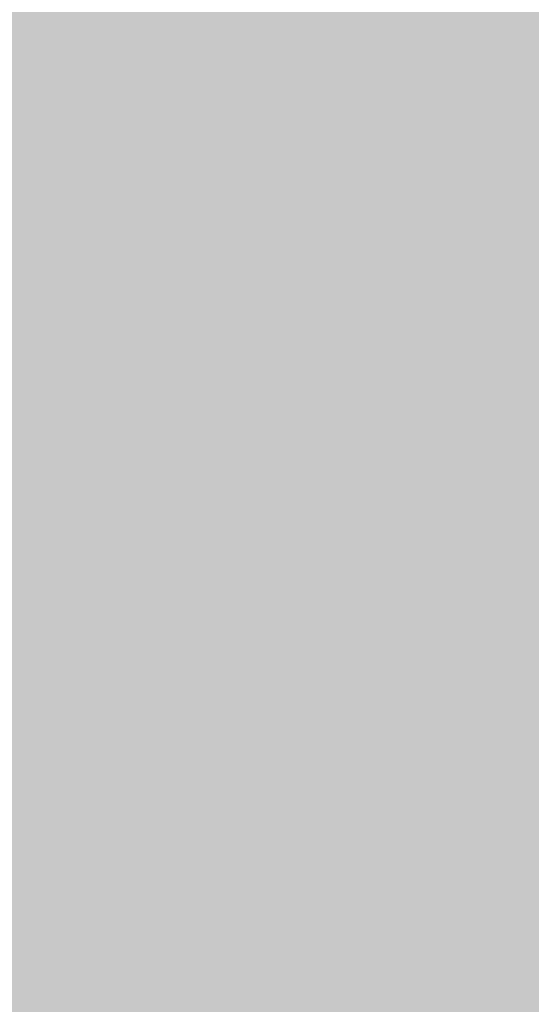
# Model space of a CAD drawing. Units: inches. Extents: x 2083 to 3317, y 1141 to 2115.
# Tile 198 of 256: x 3126.6699 to 3126.939, y 1263.6134 to 1264.1307. Entities that reach past the tile are written whole.
import ezdxf

# ---------------------------------------------------------------- set-up
doc = ezdxf.new("R2010")
doc.units = ezdxf.units.IN
doc.layers.add('A-ANNO-DIMS', color=2, linetype='Continuous', lineweight=18)
doc.layers.add('A-WALL-PATT', color=251, linetype='Continuous', lineweight=13, true_color=0x636466)
doc.styles.get("Standard").update_dxf_attribs({"font": 'arial.ttf'})
doc.dimstyles.new('ISO-25', dxfattribs={"dimtxt": 12, "dimasz": 12, "dimexe": 1.25, "dimexo": 0.625, "dimtad": 1, "dimlunit": 3, "dimtxsty": 'Standard', "dimcen": 2.5, "dimadec": 0, "dimazin": 0, "dimtfac": 1, "dimtmove": 0, "dimatfit": 3, "dimfxl": 1, "dimarcsym": 0})

# ---------------------------------------------------------------- blocks, each defined once
blk = doc.blocks.new('*D26')
at = {"layer": 'A-ANNO-DIMS', "color": 0, "lineweight": -2, "transparency": 16777216}
for p, q in [((3088.98584, 1274.91509), (3088.98584, 1270.95196)), ((3111.24004, 1274.91509), (3111.24004, 1270.95196)), ((3076.98584, 1272.20196), (2840.26245, 1272.20196)), ((3111.24004, 1272.20196), (3088.98584, 1272.20196)), ((3123.24004, 1272.20196), (3135.24004, 1272.20196))]:
    blk.add_line(p, q, dxfattribs=at)
at = {"layer": 'A-ANNO-DIMS', "color": 0, "transparency": 16777216}
for points in [[(3076.98584, 1274.20196), (3076.98584, 1270.20196), (3088.98584, 1272.20196)], [(3123.24004, 1274.20196), (3123.24004, 1270.20196), (3111.24004, 1272.20196)]]:
    blk.add_solid(points, dxfattribs=at)
at = {"layer": 'Defpoints', "color": 0, "transparency": 16777216}
for p in [(3088.98584, 1275.54009), (3111.24004, 1275.54009), (3088.98584, 1272.20196)]:
    blk.add_point(p, dxfattribs=at)
at = {"layer": 'A-ANNO-DIMS', "color": 0, "transparency": 16777216, "insert": (2952.62415, 1279.0316), "char_height": 12, "attachment_point": 5}
blk.add_mtext('NIGHTSTAND 1\'-10 1/2" TYP.', dxfattribs=at)
blk = doc.blocks.new('*D27')
at = {"layer": 'A-ANNO-DIMS', "color": 0, "lineweight": -2, "transparency": 16777216}
for p, q in [((3114.57817, 1309.79428), (3114.57817, 1321.79428)), ((3111.86504, 1297.79428), (3115.82817, 1297.79428)), ((3114.57817, 1297.79428), (3114.57817, 1275.54009)), ((3111.86504, 1275.54009), (3115.82817, 1275.54009)), ((3114.57817, 1263.54009), (3114.57817, 1140.98859))]:
    blk.add_line(p, q, dxfattribs=at)
at = {"layer": 'A-ANNO-DIMS', "color": 0, "transparency": 16777216}
for points in [[(3112.57817, 1309.79428), (3116.57817, 1309.79428), (3114.57817, 1297.79428)], [(3112.57817, 1263.54009), (3116.57817, 1263.54009), (3114.57817, 1275.54009)]]:
    blk.add_solid(points, dxfattribs=at)
at = {"layer": 'Defpoints', "color": 0, "transparency": 16777216}
for p in [(3111.24004, 1297.79428), (3111.24004, 1275.54009), (3114.57817, 1275.54009)]:
    blk.add_point(p, dxfattribs=at)
at = {"layer": 'A-ANNO-DIMS', "color": 0, "transparency": 16777216, "insert": (3107.74853, 1196.26434), "char_height": 12, "attachment_point": 5, "rotation": 90}
blk.add_mtext('1\'-10 1/2" TYP.', dxfattribs=at)

msp = doc.modelspace()

# ---------------------------------------------------------------- hatches: boundary and pattern name
at = {"layer": 'A-WALL-PATT'}
h = msp.add_hatch(color=256, dxfattribs=at)
h.dxf.hatch_style = 1
h.paths.add_polyline_path([(3126.95978, 2020.76136), (2748.95978, 2020.76136), (2604.95978, 2020.76136), (2226.95978, 2020.76136), (2226.95978, 1702.76136), (2466.95978, 1702.76136), (2466.95978, 1582.76136), (2418.95978, 1582.76136), (2418.95978, 1477.76136), (2226.95978, 1477.76136), (2226.95978, 1263.26136), (2544.95978, 1263.26136), (2544.95978, 1411.76136), (2604.95978, 1411.76136), (2685.95978, 1411.76136), (2685.95978, 1420.76136), (2604.95978, 1420.76136), (2604.95978, 1573.76136), (2604.95978, 1702.76136), (2604.95978, 2011.76136), (2748.95978, 2011.76136), (2748.95978, 1702.76136), (2862.95978, 1702.76136), (2862.95978, 1621.76136), (2871.95978, 1621.76136), (2871.95978, 1702.76136), (2883.95978, 1702.76136), (2883.95978, 1706.93946, -0.026459), (2883.95978, 1711.76136), (2757.95978, 1711.76136), (2757.95978, 1807.76136), (2787.95978, 1807.76136), (2787.95978, 1812.26136), (2757.95978, 1812.26136), (2757.95978, 2011.76136), (2877.95978, 2011.76136), (2877.95978, 1812.26136), (2847.95978, 1812.26136), (2847.95978, 1807.76136), (2889.83574, 1807.76136), (2889.83574, 1812.26136), (2882.45978, 1812.26136), (2882.45978, 2011.76136), (3117.95978, 2011.76136), (3117.95978, 1812.26136), (2937.83574, 1812.26136), (2937.83574, 1807.76136), (2995.70978, 1807.76136), (2995.70978, 1796.11767), (3000.20978, 1796.11767), (3000.20978, 1807.76136), (3117.95978, 1807.76136), (3117.95978, 1711.76136), (3000.20978, 1711.76136), (3000.20978, 1760.11767), (2998.5727, 1760.11767, -0.020711), (2995.70978, 1760.11767), (2995.70978, 1711.76136), (2931.95978, 1711.76136), (2931.95978, 1702.76136), (3126.95978, 1702.76136)])
h.paths.add_polyline_path([(2471.45978, 2011.76136), (2471.45978, 1810.01136), (2462.71694, 1810.01136), (2462.71694, 1805.51136), (2505.95978, 1805.51136), (2505.95978, 1810.01136), (2475.95978, 1810.01136), (2475.95978, 2011.76136), (2595.95978, 2011.76136), (2595.95978, 1810.01136), (2565.95978, 1810.01136), (2565.95978, 1805.51136), (2595.95978, 1805.51136), (2595.95978, 1711.76136), (2235.95978, 1711.76136), (2235.95978, 1805.51136), (2353.70978, 1805.51136), (2353.70978, 1796.05416), (2358.20978, 1796.05416), (2358.20978, 1805.51136), (2414.71694, 1805.51136), (2414.71694, 1810.01136), (2235.95978, 1810.01136), (2235.95978, 2011.76136)], flags=16)
h.paths.add_polyline_path([(2270.20473, 1994.61001), (2270.20473, 1970.61001), (2246.20473, 1970.61001), (2246.20473, 1994.61001)], flags=0)
edge = h.paths.add_edge_path(flags=0)
edge.add_ellipse((2332.02739, 1899.79818), major_axis=(-3.04299, 3.04299), ratio=0.1682525, start_angle=-161.33217, end_angle=-156.30711, ccw=False)
edge.add_ellipse((2333.08204, 1898.74353), major_axis=(-1.05465, 1.05465), ratio=0.4535321, start_angle=-123.37102, end_angle=-94.15911)
edge = h.paths.add_edge_path(flags=0)
edge.add_ellipse((2332.02739, 1968.87629), major_axis=(3.04299, 3.04299), ratio=0.1682525, start_angle=18.66783, end_angle=23.69289)
edge.add_spline(control_points=[(2332.9256, 1970.6911), (2332.22677, 1970.3361), (2330.89371, 1969.65891), (2328.41308, 1970.93214), (2327.20393, 1967.74871), (2324.7096, 1969.95559), (2322.53282, 1967.01235), (2320.01285, 1971.29581), (2317.68031, 1968.15784), (2316.04053, 1967.10205), (2315.4269, 1966.8096)], knot_values=[0, 0, 0, 0, 2.267059, 4.324559, 6.685584, 8.878641, 11.121502, 14.300359, 17.755284, 19.732645, 19.732645, 19.732645, 19.732645], degree=3, periodic=0)
edge.add_ellipse((2332.02739, 1968.87629), major_axis=(3.04299, 3.04299), ratio=0.1682525, start_angle=18.66783, end_angle=23.69289, ccw=False)
edge.add_ellipse((2333.08204, 1969.93094), major_axis=(1.05465, 1.05465), ratio=0.4535321, start_angle=56.62898, end_angle=85.84089, ccw=False)
edge = h.paths.add_edge_path(flags=0)
edge.add_spline(control_points=[(2296.42829, 1967.98791), (2293.6278, 1965.33631), (2287.70362, 1959.72709), (2299.74386, 1949.9957), (2294.53259, 1935.66853), (2290.57323, 1920.60351), (2293.39412, 1909.97369), (2296.18541, 1904.96654)], knot_values=[0.099185, 0.099185, 0.099185, 0.099185, 0.345301, 0.619822, 0.982653, 1.386093, 1.810555, 1.810555, 1.810555, 1.810555], degree=3, periodic=0)
edge.add_spline(control_points=[(2296.18541, 1904.96654), (2297.38358, 1902.6193), (2298.00097, 1901.94931), (2298.55297, 1901.46815)], knot_values=[0.006246, 0.006246, 0.006246, 0.006246, 0.055476, 0.055476, 0.055476, 0.055476], degree=3, periodic=0)
edge.add_spline(control_points=[(2298.55297, 1901.46815), (2297.25861, 1900.92322), (2295.22529, 1900.23213), (2293.06023, 1900.61421), (2292.10142, 1900.78841), (2292.08958, 1900.79057)], knot_values=[0.312835, 0.312835, 0.312835, 0.312835, 0.40178, 0.474987, 0.475903, 0.475903, 0.475903, 0.475903], degree=3, periodic=0)
edge.add_arc((2292.79365, 1904.66411), 3.93701, 215.4209, 259.69818, ccw=False)
edge.add_spline(control_points=[(2289.58531, 1902.3823), (2289.47665, 1902.53509), (2289.36848, 1902.68804), (2289.26086, 1902.84117)], knot_values=[0.102872, 0.102872, 0.102872, 0.102872, 0.116896, 0.116896, 0.116896, 0.116896], degree=3, periodic=0)
edge.add_spline(control_points=[(2289.26086, 1902.84117), (2288.6866, 1902.55019), (2287.64005, 1902.0199), (2285.88134, 1901.87395), (2283.85297, 1901.50435), (2281.71999, 1899.71054), (2278.46699, 1899.49294), (2276.15714, 1901.8832), (2272.25895, 1899.80407), (2267.77761, 1901.84318), (2262.24388, 1900.18403), (2257.41493, 1901.78206), (2254.31837, 1900.72612), (2253.17828, 1900.33734)], knot_values=[0, 0, 0, 0, 1.907977, 3.477176, 5.261074, 7.972851, 11.680248, 13.717921, 16.939592, 22.789562, 27.502503, 33.595215, 37.145618, 37.145618, 37.145618, 37.145618], degree=3, periodic=0)
edge.add_line((2253.17828, 1900.33734), (2250.24424, 1902.84117))
edge.add_line((2250.24424, 1902.84117), (2250.24424, 1965.8333))
edge.add_line((2250.24424, 1965.8333), (2253.17828, 1968.33712))
edge.add_spline(control_points=[(2253.17828, 1968.33712), (2254.31837, 1967.94835), (2257.41493, 1966.89241), (2262.24388, 1968.49043), (2267.77761, 1966.83128), (2271.52673, 1968.53722), (2273.87591, 1967.82829), (2274.2067, 1967.72764)], knot_values=[0, 0, 0, 0, 0.09018, 0.244935, 0.364644, 0.513233, 0.537855, 0.537855, 0.537855, 0.537855], degree=3, periodic=0)
edge.add_arc((2274.35289, 1963.79335), 3.93701, 72.05113, 92.12795, ccw=False)
edge.add_arc((2281.29693, 1985.23), 18.5963, 252.051134, 288.565722)
edge.add_arc((2292.31672, 1956.02888), 12.64608, 71.026788, 113.778218, ccw=False)
edge = h.paths.add_edge_path(flags=0)
edge.add_spline(control_points=[(2274.89941, 1951.85619), (2275.06616, 1951.61659), (2275.23269, 1951.37659), (2275.39799, 1951.13585)], knot_values=[1.409916, 1.409916, 1.409916, 1.409916, 1.43159, 1.43159, 1.43159, 1.43159], degree=3, periodic=0)
edge.add_spline(control_points=[(2275.39799, 1951.13585), (2275.79211, 1950.56189), (2276.17923, 1949.98377), (2276.54555, 1949.3971)], knot_values=[1.358238, 1.358238, 1.358238, 1.358238, 1.409916, 1.409916, 1.409916, 1.409916], degree=3, periodic=0)
edge.add_line((2276.54555, 1949.3971), (2277.43729, 1947.86218))
edge.add_spline(control_points=[(2277.43729, 1947.86218), (2276.30383, 1945.67311), (2274.6397, 1942.42688), (2274.63161, 1938.0939), (2272.79912, 1930.85155), (2274.35643, 1943.89705), (2275.94768, 1947.92336), (2276.54555, 1949.3971)], knot_values=[0.005632, 0.005632, 0.005632, 0.005632, 0.186014, 0.266002, 0.357087, 0.59639, 0.739732, 0.739732, 0.739732, 0.739732], degree=3, periodic=0)
edge.add_spline(control_points=[(2276.54555, 1949.3971), (2276.17923, 1949.98377), (2275.79211, 1950.56189), (2275.39799, 1951.13585)], knot_values=[1.358238, 1.358238, 1.358238, 1.358238, 1.409916, 1.409916, 1.409916, 1.409916], degree=3, periodic=0)
edge.add_spline(control_points=[(2275.39799, 1951.13585), (2274.9425, 1950.08045), (2274.20776, 1948.02527), (2273.9346, 1944.85148), (2272.46853, 1937.62749), (2273.46622, 1945.69647), (2274.70062, 1951.05947), (2274.89941, 1951.85619)], knot_values=[0.104364, 0.104364, 0.104364, 0.104364, 0.189636, 0.269624, 0.36071, 0.600013, 0.644622, 0.644622, 0.644622, 0.644622], degree=3, periodic=0)
h.paths.add_polyline_path([(2269.16751, 1963.12757, -0.357527), (2268.17063, 1960.97637, -0.092561), (2268.17063, 1939.43632, -0.357527), (2269.16751, 1937.28512, -0.357527), (2267.01631, 1938.282, -0.164785), (2254.68558, 1938.282, -0.357527), (2252.53438, 1937.28512, -0.357527), (2253.53126, 1939.43632, -0.092561), (2253.53126, 1960.97637, -0.357527), (2252.53438, 1963.12757, -0.357527), (2254.68558, 1962.13069, -0.164785), (2267.01631, 1962.13069, -0.357527)], flags=0)
h.paths.add_polyline_path([(2248.87407, 1967.8018), (2248.87407, 1957.02771), (2249.45778, 1957.02771), (2249.45778, 1911.64676), (2248.87407, 1911.64676), (2248.87407, 1900.87267), (2246.51186, 1900.87267, 0.197327), (2244.14966, 1902.45687), (2244.14966, 1966.21759, 0.197327), (2246.51186, 1967.8018)], flags=0)
h.paths.add_polyline_path([(2269.16751, 1931.38934, -0.357527), (2268.17063, 1929.23814, -0.092561), (2268.17063, 1907.6981, -0.357527), (2269.16751, 1905.54689, -0.357527), (2267.01631, 1906.54377, -0.164785), (2254.68558, 1906.54377, -0.357527), (2252.53438, 1905.54689, -0.357527), (2253.53126, 1907.6981, -0.092561), (2253.53126, 1929.23814, -0.357527), (2252.53438, 1931.38934, -0.357527), (2254.68558, 1930.39246, -0.164785), (2267.01631, 1930.39246, -0.357527)], flags=0)
edge = h.paths.add_edge_path(flags=0)
edge.add_spline(control_points=[(2276.19686, 1906.7237), (2276.16814, 1909.02893), (2276.11405, 1913.37185), (2270.59842, 1924.92498), (2273.90517, 1919.01278), (2275.92171, 1916.26206), (2275.47457, 1912.40215), (2277.25787, 1910.38062), (2276.69604, 1908.22504), (2276.64622, 1906.81302), (2276.61782, 1906.00841)], knot_values=[0, 0, 0, 0, 8.61026, 16.221274, 18.843057, 23.804898, 27.440828, 29.356102, 31.203478, 33.650687, 33.650687, 33.650687, 33.650687], degree=3, periodic=0)
edge.add_spline(control_points=[(2276.61782, 1906.00841), (2276.62331, 1905.62414), (2276.49774, 1904.62866), (2275.44178, 1903.85473), (2274.93731, 1903.08045), (2274.85908, 1902.84117)], knot_values=[0.156488, 0.156488, 0.156488, 0.156488, 0.184398, 0.231376, 0.250598, 0.250598, 0.250598, 0.250598], degree=3, periodic=0)
edge.add_line((2274.85908, 1902.84117), (2276.50598, 1902.84117))
edge.add_spline(control_points=[(2276.50598, 1902.84117), (2276.78831, 1903.08494), (2277.66507, 1904.1252), (2278.24954, 1904.34074), (2277.65387, 1908.52739), (2278.15567, 1906.22781), (2278.10046, 1905.28595), (2278.84667, 1904.06901), (2277.85679, 1903.41495), (2277.87419, 1902.99105), (2277.90356, 1902.84117)], knot_values=[0.059574, 0.059574, 0.059574, 0.059574, 0.080753, 0.103741, 0.16972, 0.176036, 0.207137, 0.240474, 0.262341, 0.27366, 0.27366, 0.27366, 0.27366], degree=3, periodic=0)
edge.add_line((2277.90356, 1902.84117), (2280.02983, 1902.84117))
edge.add_spline(control_points=[(2280.02983, 1902.84117), (2279.88822, 1903.0884), (2279.49926, 1903.98155), (2280.15228, 1905.93935), (2278.10362, 1909.65776), (2279.76239, 1907.18529), (2280.3279, 1904.87486), (2280.48511, 1903.48959), (2281.46327, 1903.24943), (2281.75834, 1902.9365), (2281.83404, 1902.84117)], knot_values=[0.013856, 0.013856, 0.013856, 0.013856, 0.034874, 0.088867, 0.107879, 0.126738, 0.158714, 0.193757, 0.217487, 0.226722, 0.226722, 0.226722, 0.226722], degree=3, periodic=0)
edge.add_spline(control_points=[(2281.83404, 1902.84117), (2281.78753, 1902.8267), (2281.64702, 1902.78299), (2281.39553, 1902.85949), (2281.08808, 1902.98524), (2280.72068, 1903.0609), (2280.33345, 1903.02573), (2280.12477, 1902.89888), (2280.02983, 1902.84117)], knot_values=[0, 0, 0, 0, 0.14413, 0.435517, 0.749276, 1.153046, 1.548371, 1.878348, 1.878348, 1.878348, 1.878348], degree=3, periodic=0)
edge.add_line((2280.02983, 1902.84117), (2277.90356, 1902.84117))
edge.add_spline(control_points=[(2277.90356, 1902.84117), (2277.89286, 1902.79586), (2277.8654, 1902.67964), (2277.60748, 1902.68748), (2277.27405, 1902.8007), (2276.83792, 1902.61977), (2276.58381, 1902.78926), (2276.50598, 1902.84117)], knot_values=[0, 0, 0, 0, 0.127189, 0.326199, 0.628009, 1.24357, 1.515331, 1.515331, 1.515331, 1.515331], degree=3, periodic=0)
edge.add_line((2276.50598, 1902.84117), (2274.85908, 1902.84117))
edge.add_spline(control_points=[(2274.85908, 1902.84117), (2274.81444, 1902.89859), (2274.72513, 1903.01345), (2274.49348, 1903.11897), (2274.24429, 1902.96054), (2273.93712, 1903.18494), (2273.61404, 1902.98314), (2273.40832, 1902.88304), (2273.32225, 1902.84117)], knot_values=[0, 0, 0, 0, 0.21843, 0.436957, 0.687977, 0.990379, 1.398396, 1.69185, 1.69185, 1.69185, 1.69185], degree=3, periodic=0)
edge.add_spline(control_points=[(2273.32225, 1902.84117), (2273.61674, 1903.44569), (2274.274, 1904.53825), (2276.02724, 1904.5737), (2276.20696, 1906.58364), (2276.19686, 1906.7237)], knot_values=[0.012227, 0.012227, 0.012227, 0.012227, 0.059472, 0.106218, 0.134458, 0.134458, 0.134458, 0.134458], degree=3, periodic=0)
h.paths.add_polyline_path([(2270.77605, 1897.78983), (2270.77605, 1873.78983), (2246.77605, 1873.78983), (2246.77605, 1897.78983)], flags=0)
h.paths.add_polyline_path([(2353.70978, 1760.00506), (2353.70978, 1760.05416), (2358.20978, 1760.05416, -0.033729)], flags=0)
h.paths.add_polyline_path([(2321.81912, 1737.52919), (2341.99533, 1737.52919, -0.414214), (2343.20327, 1736.32124), (2343.20327, 1721.0206, -0.414214), (2341.99533, 1719.81265), (2321.81912, 1719.81265, -0.414214), (2320.61117, 1721.0206), (2320.61117, 1736.32124, -0.414214)], flags=0)
h.paths.add_polyline_path([(2324.23501, 1736.32124), (2339.57944, 1736.32124, -0.414214), (2341.99533, 1733.90535), (2341.99533, 1725.44973, -0.414214), (2339.57944, 1723.03384), (2333.68059, 1723.03384), (2333.84532, 1722.04547, -0.870646), (2335.4254, 1721.82589, -0.767327), (2333.92269, 1721.42324), (2331.29102, 1721.42324, -0.767327), (2329.78832, 1721.82589, -0.870646), (2331.3684, 1722.04547), (2331.53313, 1723.03384), (2324.23501, 1723.03384, -0.414214), (2321.81912, 1725.44973), (2321.81912, 1733.90535, -0.414214)], flags=0)
h.paths.add_polyline_path([(2570.48379, 1928.61544), (2589.68379, 1928.61544), (2590.16883, 1928.61544), (2590.16883, 1904.9934), (2570.48379, 1904.9934)], flags=0)
h.paths.add_polyline_path([(2574.44732, 1927.26382, -1), (2572.82884, 1927.26382, -1)], flags=0)
h.paths.add_polyline_path([(2573.08987, 1926.94088), (2573.92503, 1927.77604), (2574.14774, 1927.55333), (2573.31258, 1926.71817)], flags=0)
h.paths.add_polyline_path([(2578.77906, 1919.72962, -1), (2571.59166, 1919.72962, -1)], flags=0)
h.paths.add_polyline_path([(2578.38536, 1919.72962, -1), (2571.98536, 1919.72962, -1)], flags=0)
h.paths.add_polyline_path([(2331.59576, 1729.47622, -1), (2333.61795, 1729.47622, -1)], flags=0)
h.paths.add_polyline_path([(2578.03423, 1927.26382, -1), (2576.41574, 1927.26382, -1)], flags=0)
h.paths.add_polyline_path([(2576.68885, 1927.53109), (2576.91156, 1927.7538), (2577.74673, 1926.91863), (2577.52402, 1926.69592)], flags=0)
h.paths.add_polyline_path([(2578.13906, 1909.85954, -1), (2572.23166, 1909.85954, -1)], flags=0)
h.paths.add_polyline_path([(2577.74536, 1909.85954, -1), (2572.62536, 1909.85954, -1)], flags=0)
h.paths.add_polyline_path([(2583.79772, 1927.26382, -1), (2582.17923, 1927.26382, -1)], flags=0)
h.paths.add_polyline_path([(2582.71865, 1927.7538), (2583.55381, 1926.91863), (2583.3311, 1926.69592), (2582.49594, 1927.53109)], flags=0)
h.paths.add_polyline_path([(2582.49594, 1927.53109), (2582.71865, 1927.7538), (2583.55381, 1926.91863), (2583.3311, 1926.69592)], flags=0)
h.paths.add_polyline_path([(2587.73906, 1920.52962, -1), (2581.83166, 1920.52962, -1)], flags=0)
h.paths.add_polyline_path([(2587.34536, 1920.52962, -1), (2582.22536, 1920.52962, -1)], flags=0)
h.paths.add_polyline_path([(2587.38462, 1927.26382, -1), (2585.76613, 1927.26382, -1)], flags=0)
h.paths.add_polyline_path([(2586.08199, 1926.98025), (2586.91716, 1927.81541), (2587.13987, 1927.5927), (2586.3047, 1926.75754)], flags=0)
h.paths.add_polyline_path([(2588.37906, 1910.65954, -1), (2581.19166, 1910.65954, -1)], flags=0)
h.paths.add_polyline_path([(2587.98536, 1910.65954, -1), (2581.58536, 1910.65954, -1)], flags=0)
h.paths.add_polyline_path([(2417.16773, 1729.4779), (2437.34394, 1729.4779, -0.414214), (2438.55188, 1728.26995), (2438.55188, 1712.96931, -0.414214), (2437.34394, 1711.76136), (2417.16773, 1711.76136, -0.414214), (2415.95978, 1712.96931), (2415.95978, 1728.26995, -0.414214)], flags=0)
h.paths.add_polyline_path([(2419.58362, 1728.26995), (2434.92805, 1728.26995, -0.414214), (2437.34394, 1725.85406), (2437.34394, 1717.39844, -0.414214), (2434.92805, 1714.98255), (2429.0292, 1714.98255), (2429.19393, 1713.99418, -0.870646), (2430.77401, 1713.7746, -0.767327), (2429.2713, 1713.37195), (2426.63963, 1713.37195, -0.767327), (2425.13693, 1713.7746, -0.870646), (2426.71701, 1713.99418), (2426.88174, 1714.98255), (2419.58362, 1714.98255, -0.414214), (2417.16773, 1717.39844), (2417.16773, 1725.85406, -0.414214)], flags=0)
h.paths.add_polyline_path([(2419.58362, 1728.26995), (2434.92805, 1728.26995, -0.414214), (2437.34394, 1725.85406), (2437.34394, 1717.39844, -0.414214), (2434.92805, 1714.98255), (2429.0292, 1714.98255), (2428.35812, 1719.00903), (2427.55282, 1719.00903), (2426.88174, 1714.98255), (2419.58362, 1714.98255, -0.414214), (2417.16773, 1717.39844), (2417.16773, 1725.85406, -0.414214)], flags=0)
h.paths.add_polyline_path([(2426.94437, 1721.42492, -1), (2428.96656, 1721.42492, -1)], flags=0)
h.paths.add_polyline_path([(2475.95978, 1702.76136), (2595.95978, 1702.76136), (2595.95978, 1582.76136), (2475.95978, 1582.76136)], flags=16)
h.paths.add_polyline_path([(2427.95978, 1573.76136), (2595.95978, 1573.76136), (2595.95978, 1468.76136), (2595.95978, 1420.76136), (2384.45978, 1420.76136), (2384.45978, 1468.76136), (2427.95978, 1468.76136)], flags=16)
h.paths.add_polyline_path([(2379.95978, 1468.76136), (2379.95978, 1420.76136), (2235.95978, 1420.76136), (2235.95978, 1468.76136)], flags=16)
h.paths.add_polyline_path([(2317.816, 1466.69577), (2337.9922, 1466.69577, -0.414214), (2339.20015, 1465.48782), (2339.20015, 1450.18718, -0.414214), (2337.9922, 1448.97923), (2317.816, 1448.97923, -0.414214), (2316.60805, 1450.18718), (2316.60805, 1465.48782, -0.414214)], flags=0)
h.paths.add_polyline_path([(2320.23189, 1465.48782), (2335.57631, 1465.48782, -0.414214), (2337.9922, 1463.07193), (2337.9922, 1454.61631, -0.414214), (2335.57631, 1452.20042), (2329.67747, 1452.20042), (2329.84219, 1451.21205, -0.870646), (2331.42228, 1450.99247, -0.767327), (2329.91957, 1450.58983), (2327.2879, 1450.58983, -0.767327), (2325.7852, 1450.99247, -0.870646), (2327.36528, 1451.21205), (2327.53001, 1452.20042), (2320.23189, 1452.20042, -0.414214), (2317.816, 1454.61631), (2317.816, 1463.07193, -0.414214)], flags=0)
h.paths.add_polyline_path([(2320.23189, 1465.48782), (2335.57631, 1465.48782, -0.414214), (2337.9922, 1463.07193), (2337.9922, 1454.61631, -0.414214), (2335.57631, 1452.20042), (2329.67747, 1452.20042), (2329.00638, 1456.22691), (2328.20109, 1456.22691), (2327.53001, 1452.20042), (2320.23189, 1452.20042, -0.414214), (2317.816, 1454.61631), (2317.816, 1463.07193, -0.414214)], flags=0)
h.paths.add_polyline_path([(2327.59264, 1458.6428, -1), (2329.61483, 1458.6428, -1)], flags=0)
h.paths.add_polyline_path([(2244.41174, 1433.34045), (2241.92094, 1433.34045, -0.414214), (2240.01786, 1435.24354), (2240.01786, 1440.95281, -0.414211), (2241.92093, 1442.8559), (2244.41174, 1442.8559, -1.976472)], flags=0)
h.paths.add_polyline_path([(2245.35689, 1434.39754, -0.414214), (2245.35689, 1441.79881, -2.144098)], flags=0)
h.paths.add_polyline_path([(2535.95978, 1416.26136), (2535.95978, 1272.26136), (2235.95978, 1272.26136), (2235.95978, 1416.26136)], flags=16)
h.paths.add_polyline_path([(2260.11956, 1384.29284), (2260.11956, 1362.03865), (2237.86537, 1362.03865), (2237.86537, 1384.29284)], flags=0)
edge = h.paths.add_edge_path(flags=0)
edge.add_line((2318.25185, 1362.0933), (2318.1458, 1362.00097))
edge.add_ellipse((2317.44512, 1360.43104), major_axis=(2.82164, 2.82164), ratio=0.1682525, start_angle=18.66783, end_angle=20.94813, ccw=False)
edge.add_ellipse((2318.42305, 1361.40897), major_axis=(0.97793, 0.97793), ratio=0.4535321, start_angle=56.62898, end_angle=70.2262, ccw=False)
edge = h.paths.add_edge_path(flags=0)
edge.add_line((2319.10737, 1295.57108), (2319.01504, 1295.67713))
edge.add_ellipse((2317.44512, 1296.37781), major_axis=(-2.82164, 2.82164), ratio=0.1682525, start_angle=-161.33217, end_angle=-159.05187, ccw=False)
edge.add_ellipse((2318.42305, 1295.39988), major_axis=(-0.97793, 0.97793), ratio=0.4535321, start_angle=-123.37102, end_angle=-109.7738)
edge = h.paths.add_edge_path(flags=0)
edge.add_spline(control_points=[(2284.21035, 1301.17022), (2284.58069, 1300.44472), (2284.89119, 1299.89202), (2285.15955, 1299.46102)], knot_values=[0.039066, 0.039066, 0.039066, 0.039066, 0.055476, 0.055476, 0.055476, 0.055476], degree=3, periodic=0)
edge.add_line((2285.15955, 1299.46102), (2284.21035, 1301.17022))
edge = h.paths.add_edge_path(flags=0)
edge.add_line((2280.41246, 1297.29801), (2283.36999, 1297.03612))
edge.add_line((2283.36999, 1297.03612), (2286.40569, 1297.92631))
edge.add_spline(control_points=[(2286.40569, 1297.92631), (2285.30549, 1297.46312), (2284.34478, 1297.12915), (2283.36999, 1297.03612)], knot_values=[0.394369, 0.394369, 0.394369, 0.394369, 0.475903, 0.475903, 0.475903, 0.475903], degree=3, periodic=0)
edge.add_spline(control_points=[(2283.36999, 1297.03612), (2283.28139, 1297.02767), (2282.31629, 1296.95734), (2281.3125, 1297.13448), (2280.42344, 1297.29602), (2280.41246, 1297.29801)], knot_values=[0.312835, 0.312835, 0.312835, 0.312835, 0.320246, 0.393453, 0.394369, 0.394369, 0.394369, 0.394369], degree=3, periodic=0)
edge = h.paths.add_edge_path(flags=0)
edge.add_line((2284.43556, 1359.60729), (2280.44629, 1355.32805))
edge.add_line((2280.44629, 1355.32805), (2279.57999, 1351.01775))
edge.add_line((2279.57999, 1351.01775), (2282.41297, 1346.58043))
edge.add_spline(control_points=[(2282.41297, 1346.58043), (2283.15333, 1345.58924), (2284.2529, 1344.0289), (2284.80104, 1342.38717), (2284.93516, 1341.80554)], knot_values=[1.240098, 1.240098, 1.240098, 1.240098, 1.332892, 1.382712, 1.382712, 1.382712, 1.382712], degree=3, periodic=0)
edge.add_spline(control_points=[(2284.93516, 1341.80554), (2285.31911, 1340.1406), (2285.23303, 1338.4092), (2284.90994, 1336.65412)], knot_values=[1.097484, 1.097484, 1.097484, 1.097484, 1.240098, 1.240098, 1.240098, 1.240098], degree=3, periodic=0)
edge.add_spline(control_points=[(2284.90994, 1336.65412), (2284.58685, 1334.89904), (2284.02675, 1333.12027), (2283.46264, 1331.36058)], knot_values=[0.95487, 0.95487, 0.95487, 0.95487, 1.097484, 1.097484, 1.097484, 1.097484], degree=3, periodic=0)
edge.add_line((2283.46264, 1331.36058), (2281.89038, 1326.15336))
edge.add_line((2281.89038, 1326.15336), (2280.75626, 1321.05609))
edge.add_line((2280.75626, 1321.05609), (2280.2992, 1316.00198))
edge.add_line((2280.2992, 1316.00198), (2280.71593, 1310.95007))
edge.add_line((2280.71593, 1310.95007), (2282.02809, 1305.97214))
edge.add_line((2282.02809, 1305.97214), (2284.21035, 1301.17022))
edge.add_spline(control_points=[(2284.21035, 1301.17022), (2283.34073, 1302.73019), (2282.6119, 1304.33649), (2282.02809, 1305.97214)], knot_values=[0.099185, 0.099185, 0.099185, 0.099185, 0.241799, 0.241799, 0.241799, 0.241799], degree=3, periodic=0)
edge.add_spline(control_points=[(2282.02809, 1305.97214), (2281.44428, 1307.60778), (2281.00549, 1309.27276), (2280.71593, 1310.95007)], knot_values=[0.241799, 0.241799, 0.241799, 0.241799, 0.384413, 0.384413, 0.384413, 0.384413], degree=3, periodic=0)
edge.add_spline(control_points=[(2280.71593, 1310.95007), (2280.43324, 1312.58761), (2280.28939, 1314.27696), (2280.29889, 1315.96203), (2280.2992, 1316.00198)], knot_values=[0.384413, 0.384413, 0.384413, 0.384413, 0.523647, 0.527028, 0.527028, 0.527028, 0.527028], degree=3, periodic=0)
edge.add_spline(control_points=[(2280.2992, 1316.00198), (2280.31233, 1317.68696), (2280.47787, 1319.36793), (2280.75626, 1321.05609)], knot_values=[0.527028, 0.527028, 0.527028, 0.527028, 0.669642, 0.669642, 0.669642, 0.669642], degree=3, periodic=0)
edge.add_spline(control_points=[(2280.75626, 1321.05609), (2281.03465, 1322.74425), (2281.42588, 1324.43961), (2281.89038, 1326.15336)], knot_values=[0.669642, 0.669642, 0.669642, 0.669642, 0.812256, 0.812256, 0.812256, 0.812256], degree=3, periodic=0)
edge.add_spline(control_points=[(2281.89038, 1326.15336), (2282.26438, 1327.53325), (2282.78787, 1329.26181), (2283.35275, 1331.01778), (2283.46264, 1331.36058)], knot_values=[0.812256, 0.812256, 0.812256, 0.812256, 0.927087, 0.95487, 0.95487, 0.95487, 0.95487], degree=3, periodic=0)
edge.add_line((2283.46264, 1331.36058), (2284.90994, 1336.65412))
edge.add_line((2284.90994, 1336.65412), (2284.93516, 1341.80554))
edge.add_line((2284.93516, 1341.80554), (2282.41297, 1346.58043))
edge.add_spline(control_points=[(2282.41297, 1346.58043), (2281.27513, 1348.10379), (2280.07845, 1349.57032), (2279.57999, 1351.01775)], knot_values=[1.382712, 1.382712, 1.382712, 1.382712, 1.525326, 1.525326, 1.525326, 1.525326], degree=3, periodic=0)
edge.add_spline(control_points=[(2279.57999, 1351.01775), (2279.44328, 1351.41472), (2279.13631, 1352.85692), (2279.73519, 1354.29039), (2280.44629, 1355.32805)], knot_values=[1.525326, 1.525326, 1.525326, 1.525326, 1.564439, 1.667941, 1.667941, 1.667941, 1.667941], degree=3, periodic=0)
edge.add_spline(control_points=[(2280.44629, 1355.32805), (2281.42611, 1356.75784), (2282.93084, 1358.18256), (2284.43556, 1359.60729)], knot_values=[1.667941, 1.667941, 1.667941, 1.667941, 1.810555, 1.810555, 1.810555, 1.810555], degree=3, periodic=0)
edge.add_arc((2280.62307, 1348.51818), 11.72618, 71.026788, 113.778218)
edge.add_arc((2270.40489, 1375.59516), 17.24357, 252.051134, 288.565722, ccw=False)
edge.add_arc((2263.96597, 1355.71785), 3.65062, 72.05113, 92.12795)
edge.add_arc((2263.96597, 1355.71785), 3.65062, 92.12795, 177.98513)
edge.add_spline(control_points=[(2260.3176, 1355.8462), (2260.26042, 1354.22067), (2260.55128, 1350.18655), (2262.99934, 1346.76625), (2264.47274, 1344.64902)], knot_values=[1.43159, 1.43159, 1.43159, 1.43159, 1.564144, 1.770695, 1.770695, 1.770695, 1.770695], degree=3, periodic=0)
edge.add_line((2264.47274, 1344.64902), (2264.93559, 1343.98253))
edge.add_spline(control_points=[(2263.80104, 1340.24811), (2263.84324, 1340.51409), (2264.06724, 1341.75647), (2264.51269, 1343.00245), (2264.93505, 1343.98108)], knot_values=[0.53657, 0.53657, 0.53657, 0.53657, 0.559349, 0.644622, 0.644622, 0.644622, 0.644622], degree=3, periodic=0)
edge.add_spline(control_points=[(2264.93505, 1343.98108), (2265.11777, 1343.71497), (2265.29888, 1343.44791), (2265.47676, 1343.17936)], knot_values=[1.384077, 1.384077, 1.384077, 1.384077, 1.409916, 1.409916, 1.409916, 1.409916], degree=3, periodic=0)
edge.add_spline(control_points=[(2265.47676, 1343.17936), (2265.65464, 1342.91082), (2265.8293, 1342.64081), (2265.99913, 1342.36881)], knot_values=[1.358238, 1.358238, 1.358238, 1.358238, 1.384077, 1.384077, 1.384077, 1.384077], degree=3, periodic=0)
edge.add_line((2265.99913, 1342.36881), (2266.82601, 1340.94555))
edge.add_spline(control_points=[(2266.82601, 1340.94555), (2268.8944, 1337.08969), (2271.39817, 1325.843), (2270.51616, 1310.56856), (2275.91938, 1301.86061), (2277.78951, 1299.19945)], knot_values=[0.116896, 0.116896, 0.116896, 0.116896, 0.472987, 1.050969, 1.313793, 1.313793, 1.313793, 1.313793], degree=3, periodic=0)
edge.add_spline(control_points=[(2277.78951, 1299.19945), (2277.83941, 1299.12845), (2277.88943, 1299.0575), (2277.93957, 1298.98658)], knot_values=[0.109884, 0.109884, 0.109884, 0.109884, 0.116896, 0.116896, 0.116896, 0.116896], degree=3, periodic=0)
edge.add_line((2277.93957, 1298.98658), (2277.78885, 1299.19911))
edge.add_spline(control_points=[(2277.78885, 1299.19911), (2277.25658, 1298.92941), (2276.28635, 1298.4379), (2275.03935, 1298.33442), (2274.38333, 1298.2389), (2274.21525, 1298.20934)], knot_values=[33.12187, 33.12187, 33.12187, 33.12187, 35.029056, 36.598255, 37.144827, 37.144827, 37.144827, 37.144827], degree=3, periodic=0)
edge.add_line((2274.21525, 1298.20934), (2273.07315, 1297.89296))
edge.add_spline(control_points=[(2273.07315, 1297.89296), (2272.32294, 1297.57978), (2271.03915, 1296.51051), (2269.24839, 1296.22606), (2268.4231, 1296.37465)], knot_values=[26.532584, 26.532584, 26.532584, 26.532584, 29.198919, 31.839101, 31.839101, 31.839101, 31.839101], degree=3, periodic=0)
edge.add_line((2268.4231, 1296.37465), (2263.8785, 1297.45753))
edge.add_spline(control_points=[(2263.8785, 1297.45753), (2263.55608, 1297.35943), (2261.86031, 1296.83869), (2260.23878, 1297.28241), (2258.93345, 1297.51646)], knot_values=[15.919551, 15.919551, 15.919551, 15.919551, 16.939592, 21.226067, 21.226067, 21.226067, 21.226067], degree=3, periodic=0)
edge.add_line((2258.93345, 1297.51646), (2254.05523, 1297.32901))
edge.add_spline(control_points=[(2254.05523, 1297.32901), (2253.75553, 1297.29582), (2252.11368, 1297.16517), (2250.46187, 1297.54422), (2249.12969, 1297.66788)], knot_values=[5.306517, 5.306517, 5.306517, 5.306517, 6.276435, 10.613034, 10.613034, 10.613034, 10.613034], degree=3, periodic=0)
edge.add_line((2249.12969, 1297.66788), (2244.33165, 1296.87776))
edge.add_line((2244.33165, 1296.87776), (2241.61103, 1299.19945))
edge.add_line((2241.61103, 1299.19945), (2241.61103, 1357.6094))
edge.add_line((2241.61103, 1357.6094), (2244.33165, 1359.9311))
edge.add_line((2244.33165, 1359.9311), (2252.72882, 1359.54269))
edge.add_spline(control_points=[(2252.72882, 1359.54269), (2252.87094, 1359.54644), (2253.30574, 1359.54817), (2253.73984, 1359.51427), (2254.03174, 1359.48243)], knot_values=[0.233291, 0.233291, 0.233291, 0.233291, 0.244935, 0.268927, 0.268927, 0.268927, 0.268927], degree=3, periodic=0)
edge.add_line((2254.03174, 1359.48243), (2259.58719, 1359.41639))
edge.add_spline(control_points=[(2259.58719, 1359.41639), (2260.67707, 1359.6285), (2262.0732, 1359.897), (2263.52369, 1359.45928), (2263.83042, 1359.36595)], knot_values=[0.422516, 0.422516, 0.422516, 0.422516, 0.513233, 0.537855, 0.537855, 0.537855, 0.537855], degree=3, periodic=0)
edge.add_arc((2263.96597, 1355.71785), 3.65062, 72.05113, 92.12795, ccw=False)
edge.add_arc((2270.40489, 1375.59516), 17.24357, 252.051134, 288.565722)
edge.add_arc((2280.62307, 1348.51818), 11.72618, 71.026788, 113.778218, ccw=False)
h.paths.add_polyline_path([(2240.34053, 1359.43471), (2240.34053, 1349.44435), (2240.88178, 1349.44435), (2240.88178, 1307.3645), (2240.34053, 1307.3645), (2240.34053, 1297.37414), (2238.15016, 1297.37414, 0.197327), (2235.95978, 1298.84311), (2235.95978, 1357.96575, 0.197327), (2238.15016, 1359.43471)], flags=0)
h.paths.add_polyline_path([(2259.15779, 1355.1005, -0.357527), (2258.23342, 1353.10578, -0.092561), (2258.23342, 1333.1326, -0.357527), (2259.15779, 1331.13788, -0.357527), (2257.16307, 1332.06225, -0.164785), (2245.7293, 1332.06225, -0.357527), (2243.73458, 1331.13788, -0.357527), (2244.65895, 1333.1326, -0.092561), (2244.65895, 1353.10578, -0.357527), (2243.73458, 1355.1005, -0.357527), (2245.7293, 1354.17613, -0.164785), (2257.16307, 1354.17613, -0.357527)], flags=0)
edge = h.paths.add_edge_path(flags=0)
edge.add_line((2265.99913, 1342.36881), (2266.82601, 1340.94555))
edge.add_line((2266.82601, 1340.94555), (2265.30756, 1337.81407))
edge.add_line((2265.30756, 1337.81407), (2264.35823, 1334.65294))
edge.add_line((2264.35823, 1334.65294), (2264.26201, 1333.7997))
edge.add_spline(control_points=[(2264.26201, 1333.7997), (2264.20836, 1333.18705), (2264.16206, 1332.36553), (2264.00714, 1331.41393), (2263.96905, 1331.20183)], knot_values=[0.464444, 0.464444, 0.464444, 0.464444, 0.516691, 0.531608, 0.531608, 0.531608, 0.531608], degree=3, periodic=0)
edge.add_spline(control_points=[(2263.96905, 1331.20183), (2263.77453, 1330.11887), (2263.42437, 1328.79084), (2263.25742, 1328.53065), (2263.23403, 1328.51461)], knot_values=[0.372682, 0.372682, 0.372682, 0.372682, 0.44885, 0.464444, 0.464444, 0.464444, 0.464444], degree=3, periodic=0)
edge.add_spline(control_points=[(2263.23403, 1328.51461), (2263.09638, 1328.42023), (2263.13117, 1329.30148), (2263.27495, 1330.61575)], knot_values=[0.280919, 0.280919, 0.280919, 0.280919, 0.372682, 0.372682, 0.372682, 0.372682], degree=3, periodic=0)
edge.add_spline(control_points=[(2263.27495, 1330.61575), (2263.41874, 1331.93002), (2263.67152, 1333.67732), (2263.96985, 1335.31503)], knot_values=[0.189157, 0.189157, 0.189157, 0.189157, 0.280919, 0.280919, 0.280919, 0.280919], degree=3, periodic=0)
edge.add_spline(control_points=[(2263.96985, 1335.31503), (2264.1005, 1336.03219), (2264.41878, 1337.62191), (2264.75485, 1338.86443), (2264.94742, 1339.49112)], knot_values=[0.097394, 0.097394, 0.097394, 0.097394, 0.137578, 0.189157, 0.189157, 0.189157, 0.189157], degree=3, periodic=0)
edge.add_spline(control_points=[(2264.94742, 1339.49112), (2265.29002, 1340.60605), (2265.64424, 1341.494), (2265.99913, 1342.36881)], knot_values=[0.005632, 0.005632, 0.005632, 0.005632, 0.097394, 0.097394, 0.097394, 0.097394], degree=3, periodic=0)
h.paths.add_polyline_path([(2259.15779, 1325.67097, -0.357527), (2258.23342, 1323.67625, -0.092561), (2258.23342, 1303.70307, -0.357527), (2259.15779, 1301.70835, -0.357527), (2257.16307, 1302.63272, -0.164785), (2245.7293, 1302.63272, -0.357527), (2243.73458, 1301.70835, -0.357527), (2244.65895, 1303.70307, -0.092561), (2244.65895, 1323.67625, -0.357527), (2243.73458, 1325.67097, -0.357527), (2245.7293, 1324.74661, -0.164785), (2257.16307, 1324.74661, -0.357527)], flags=0)
edge = h.paths.add_edge_path(flags=0)
edge.add_spline(control_points=[(2261.70894, 1317.31142), (2261.67948, 1317.41758), (2261.76186, 1317.38853), (2262.49074, 1316.08987), (2262.96218, 1315.3009)], knot_values=[14.955861, 14.955861, 14.955861, 14.955861, 16.221274, 18.694826, 18.694826, 18.694826, 18.694826], degree=3, periodic=0)
edge.add_spline(control_points=[(2262.96218, 1315.3009), (2262.99044, 1315.25362), (2263.7021, 1314.06738), (2264.34898, 1313.12715), (2264.73005, 1312.16415)], knot_values=[18.694826, 18.694826, 18.694826, 18.694826, 18.843057, 22.433791, 22.433791, 22.433791, 22.433791], degree=3, periodic=0)
edge.add_spline(control_points=[(2264.73005, 1312.16415), (2264.87556, 1311.79644), (2265.17687, 1310.76981), (2265.14307, 1309.55926), (2265.24774, 1308.82419)], knot_values=[22.433791, 22.433791, 22.433791, 22.433791, 23.804898, 26.172756, 26.172756, 26.172756, 26.172756], degree=3, periodic=0)
edge.add_line((2265.24774, 1308.82419), (2265.85077, 1307.17189))
edge.add_spline(control_points=[(2265.85077, 1307.17189), (2266.06502, 1306.82168), (2266.38439, 1306.33225), (2266.4244, 1305.78055), (2266.42037, 1305.61122)], knot_values=[28.062562, 28.062562, 28.062562, 28.062562, 29.356102, 29.911721, 29.911721, 29.911721, 29.911721], degree=3, periodic=0)
edge.add_spline(control_points=[(2266.42037, 1305.61122), (2266.41612, 1305.43259), (2266.394, 1305.25), (2266.36478, 1305.06586)], knot_values=[29.911721, 29.911721, 29.911721, 29.911721, 30.497837, 30.497837, 30.497837, 30.497837], degree=3, periodic=0)
edge.add_line((2266.36478, 1305.06586), (2266.06615, 1302.1363))
edge.add_spline(control_points=[(2266.06615, 1302.1363), (2266.07124, 1301.77998), (2265.99808, 1301.19998), (2265.66327, 1300.75896), (2265.50891, 1300.58588)], knot_values=[0.156488, 0.156488, 0.156488, 0.156488, 0.184398, 0.203543, 0.203543, 0.203543, 0.203543], degree=3, periodic=0)
edge.add_line((2265.50891, 1300.58588), (2264.43534, 1299.19945))
edge.add_line((2264.43534, 1299.19945), (2265.96244, 1299.19945))
edge.add_line((2265.96244, 1299.19945), (2267.33599, 1301.17528))
edge.add_line((2267.33599, 1301.17528), (2267.31167, 1301.98624))
edge.add_spline(control_points=[(2267.31167, 1301.98624), (2267.26111, 1302.8624), (2267.16021, 1303.73713), (2267.27149, 1303.3259)], knot_values=[0.126229, 0.126229, 0.126229, 0.126229, 0.166617, 0.166617, 0.166617, 0.166617], degree=3, periodic=0)
edge.add_spline(control_points=[(2267.27149, 1303.3259), (2267.28003, 1303.2943), (2267.30979, 1303.17537), (2267.37345, 1302.88361), (2267.40612, 1302.68283), (2267.41793, 1302.60103)], knot_values=[0.166617, 0.166617, 0.166617, 0.166617, 0.16972, 0.176036, 0.180765, 0.180765, 0.180765, 0.180765], degree=3, periodic=0)
edge.add_spline(control_points=[(2267.74389, 1300.9875), (2267.68758, 1301.15094), (2267.48052, 1301.65666), (2267.48375, 1302.14479), (2267.41793, 1302.60103)], knot_values=[0.180765, 0.180765, 0.180765, 0.180765, 0.193767, 0.220139, 0.220139, 0.220139, 0.220139], degree=3, periodic=0)
edge.add_line((2267.41793, 1302.60103), (2267.74389, 1300.9875))
edge.add_spline(control_points=[(2267.74389, 1300.9875), (2267.83196, 1300.73188), (2267.93202, 1300.3099), (2267.55484, 1299.97452), (2267.42937, 1299.82921)], knot_values=[0.220139, 0.220139, 0.220139, 0.220139, 0.240474, 0.25489, 0.25489, 0.25489, 0.25489], degree=3, periodic=0)
edge.add_line((2267.42937, 1299.82921), (2267.25836, 1299.19945))
edge.add_line((2267.25836, 1299.19945), (2269.22996, 1299.19945))
edge.add_spline(control_points=[(2269.22996, 1299.19945), (2269.09865, 1299.42869), (2268.84277, 1300.01625), (2269.01157, 1300.91592), (2268.9468, 1301.66074)], knot_values=[0.013856, 0.013856, 0.013856, 0.013856, 0.034874, 0.067073, 0.067073, 0.067073, 0.067073], degree=3, periodic=0)
edge.add_line((2268.9468, 1301.66074), (2268.43158, 1303.60311))
edge.add_spline(control_points=[(2268.43158, 1303.60311), (2268.1756, 1304.19237), (2267.59621, 1305.2513), (2268.0407, 1304.62321), (2268.25139, 1304.28242)], knot_values=[0.090155, 0.090155, 0.090155, 0.090155, 0.107879, 0.120289, 0.120289, 0.120289, 0.120289], degree=3, periodic=0)
edge.add_spline(control_points=[(2268.25139, 1304.28242), (2268.36088, 1304.10533), (2269.05775, 1302.91798), (2269.38269, 1301.59042), (2269.52141, 1300.77593), (2269.57522, 1300.55578)], knot_values=[0.120289, 0.120289, 0.120289, 0.120289, 0.126738, 0.158714, 0.173506, 0.173506, 0.173506, 0.173506], degree=3, periodic=0)
edge.add_line((2269.57522, 1300.55578), (2270.6858, 1299.42126))
edge.add_spline(control_points=[(2270.6858, 1299.42126), (2270.76722, 1299.35725), (2270.83785, 1299.2814), (2270.90292, 1299.19945)], knot_values=[0.21816, 0.21816, 0.21816, 0.21816, 0.226722, 0.226722, 0.226722, 0.226722], degree=3, periodic=0)
edge.add_line((2270.9372, 1299.19291), (2270.90292, 1299.19945))
edge.add_spline(control_points=[(2270.90292, 1299.19945), (2270.85981, 1299.18603), (2270.72951, 1299.1455), (2270.49631, 1299.21644), (2270.27166, 1299.30832), (2270.12102, 1299.34796), (2270.06334, 1299.35956)], knot_values=[0.939174, 0.939174, 0.939174, 0.939174, 1.083304, 1.374691, 1.68845, 1.878348, 1.878348, 1.878348, 1.878348], degree=3, periodic=0)
edge.add_line((2270.06334, 1299.35956), (2269.22996, 1299.19945))
edge.add_line((2269.22996, 1299.19945), (2267.25836, 1299.19945))
edge.add_spline(control_points=[(2267.25836, 1299.19945), (2267.24843, 1299.15743), (2267.22297, 1299.04967), (2266.98382, 1299.05694), (2266.80921, 1299.11623), (2266.6769, 1299.10909), (2266.63653, 1299.10481)], knot_values=[0.757665, 0.757665, 0.757665, 0.757665, 0.884854, 1.083864, 1.385675, 1.515331, 1.515331, 1.515331, 1.515331], degree=3, periodic=0)
edge.add_spline(control_points=[(2266.63653, 1299.10481), (2266.48522, 1299.08879), (2266.23581, 1299.01712), (2266.03461, 1299.15132), (2265.96244, 1299.19945)], knot_values=[0, 0, 0, 0, 0.485905, 0.757665, 0.757665, 0.757665, 0.757665], degree=3, periodic=0)
edge.add_line((2265.96244, 1299.19945), (2264.43534, 1299.19945))
edge.add_line((2264.43534, 1299.19945), (2263.85844, 1299.36712))
edge.add_spline(control_points=[(2263.85844, 1299.36712), (2263.81894, 1299.37091), (2263.77953, 1299.38572), (2263.74013, 1299.4015)], knot_values=[0.845925, 0.845925, 0.845925, 0.845925, 0.978627, 0.978627, 0.978627, 0.978627], degree=3, periodic=0)
edge.add_line((2263.72179, 1299.39643), (2263.01031, 1299.19945))
edge.add_spline(control_points=[(2263.01031, 1299.19945), (2263.24579, 1299.68286), (2263.50603, 1300.12811), (2263.87349, 1300.40803)], knot_values=[0.012227, 0.012227, 0.012227, 0.012227, 0.052971, 0.052971, 0.052971, 0.052971], degree=3, periodic=0)
edge.add_spline(control_points=[(2263.87349, 1300.40803), (2263.93213, 1300.4527), (2264.08424, 1300.55298), (2264.25519, 1300.62422), (2264.35969, 1300.66475)], knot_values=[0.052971, 0.052971, 0.052971, 0.052971, 0.059472, 0.069086, 0.069086, 0.069086, 0.069086], degree=3, periodic=0)
edge.add_line((2264.35969, 1300.66475), (2265.1419, 1301.07777))
edge.add_line((2265.1419, 1301.07777), (2265.67581, 1302.79956))
edge.add_line((2265.67581, 1302.79956), (2265.5407, 1305.70407))
edge.add_line((2265.5407, 1305.70407), (2264.80307, 1309.32772))
edge.add_line((2264.80307, 1309.32772), (2263.04053, 1314.09179))
edge.add_spline(control_points=[(2263.04053, 1314.09179), (2262.38357, 1315.67144), (2261.79597, 1316.99775), (2261.70894, 1317.31142)], knot_values=[11.216896, 11.216896, 11.216896, 11.216896, 14.955861, 14.955861, 14.955861, 14.955861], degree=3, periodic=0)
h.paths.add_polyline_path([(2871.95978, 1416.26136), (2895.91005, 1416.26136), (2895.91005, 1420.76136), (2871.95978, 1420.76136), (2871.95978, 1501.76136), (2862.95978, 1501.76136), (2862.95978, 1420.76136), (2805.95978, 1420.76136), (2805.95978, 1411.76136), (2862.95978, 1411.76136), (2862.95978, 1263.26136), (3126.95978, 1263.26136), (3126.95978, 1411.76136), (3126.95978, 1486.76136), (2943.95978, 1486.76136), (2943.95978, 1477.76136), (2967.86031, 1477.76136), (2967.86031, 1420.76136), (2943.91005, 1420.76136), (2943.91005, 1416.26136), (3117.95978, 1416.26136), (3117.95978, 1420.76136), (2972.36031, 1420.76136), (2972.36031, 1477.76136), (3117.95978, 1477.76136), (3117.95978, 1420.76136), (3117.95978, 1272.26136), (2871.95978, 1272.26136)], flags=0)
h.paths.add_polyline_path([(2457.12563, 1485.94251), (2527.60265, 1485.94251), (2527.60265, 1537.6357), (2457.12563, 1537.6357)], flags=8)
h.paths.add_polyline_path([(2481.00506, 1609.9818), (2590.76582, 1609.9818), (2590.76582, 1682.00336), (2481.00506, 1682.00336)], flags=8)
h.paths.add_polyline_path([(2483.08502, 1729.12678), (2553.56205, 1729.12678), (2553.56205, 1780.81998), (2483.08502, 1780.81998)], flags=8)
h = msp.add_hatch(color=256, dxfattribs=at)
h.dxf.hatch_style = 1
h.paths.add_polyline_path([(3126.95978, 1486.76136), (2943.95978, 1486.76136), (2943.95978, 1477.76136), (2967.86031, 1477.76136), (2967.86031, 1420.76136), (2943.91005, 1420.76136), (2943.91005, 1416.26136), (3117.95978, 1416.26136), (3117.95978, 1420.76136), (2972.36031, 1420.76136), (2972.36031, 1477.76136), (3117.95978, 1477.76136), (3117.95978, 1420.76136), (3117.95978, 1272.26136), (2871.95978, 1272.26136), (2871.95978, 1416.26136), (2895.91005, 1416.26136), (2895.91005, 1420.76136), (2871.95978, 1420.76136), (2871.95978, 1501.76136), (2862.95978, 1501.76136), (2862.95978, 1420.76136), (2805.95978, 1420.76136), (2805.95978, 1411.76136), (2862.95978, 1411.76136), (2862.95978, 1263.26136), (3126.95978, 1263.26136), (3126.95978, 1411.76136)])

# ---------------------------------------------------------------- dimensions: what is measured, and where the dimension line sits
at = {"layer": 'A-ANNO-DIMS'}
for base, p1, p2, angle, text, picture, middle in [((3114.57817, 1275.54009), (3111.24004, 1297.79428), (3111.24004, 1275.54009), 270, '<> TYP.', '*D27', (3107.74853, 1196.26434)), ((3088.98584, 1272.20196), (3111.24004, 1275.54009), (3088.98584, 1275.54009), 180, 'NIGHTSTAND <> TYP.', '*D26', (2952.62415, 1279.0316))]:
    dim = msp.add_linear_dim(base=base, p1=p1, p2=p2, angle=angle, text=text, dimstyle='ISO-25', override={"dimdec": 1, "dimlfac": 1, "dimrnd": 0, "dimzin": 1, "dimdsep": 46, "dimlunit": 4, "dimfrac": 2}, dxfattribs=at)
    dim.commit()
    dim.dimension.update_dxf_attribs({"geometry": picture, "text_midpoint": middle})

doc.saveas('drawing.dxf')
